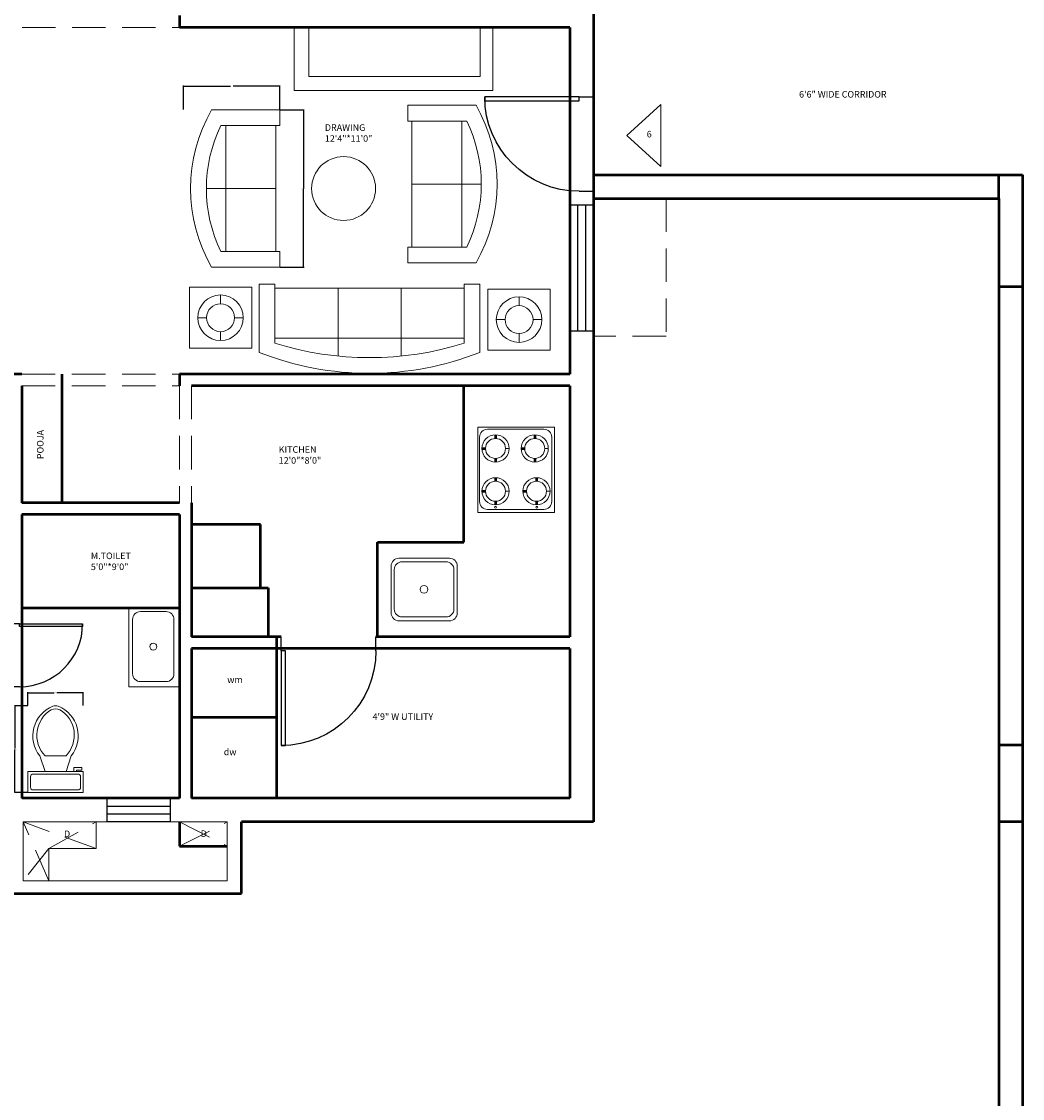
# Model space of a CAD drawing. Units: inches. Extents: x 4795 to 6024, y 2716 to 5025.
# Tile 10 of 19: x 5069 to 5450, y 3816 to 4226. Entities that reach past the tile are written whole.
import ezdxf

# ---------------------------------------------------------------- set-up
doc = ezdxf.new("R2010")
doc.units = ezdxf.units.IN
doc.linetypes.add('DASHED', pattern=[19.05, 12.7, -6.35])
for name, color, linetype, lineweight in [('A-ANNO-DIMS', 2, 'Continuous', 18), ('A-ANNO-TEXT', 7, 'Continuous', 18), ('A-AREA-IDEN', 3, 'Continuous', 18), ('A-DOOR', 4, 'Continuous', 25), ('A-FLOR-FIXT', 9, 'Continuous', 18), ('A-FURN', 8, 'Continuous', 18), ('A-GLAZ', 4, 'Continuous', 25), ('A-WALL', 7, 'Continuous', 50), ('A-WALL-OVHD', 8, 'DASHED', 18)]:
    doc.layers.add(name, color=color, linetype=linetype, lineweight=lineweight)
doc.styles.get("Standard").update_dxf_attribs({"font": 'arial.ttf'})
doc.dimstyles.get("Standard").update_dxf_attribs({"dimtxt": 0.18, "dimasz": 0.18, "dimexe": 0.18, "dimexo": 0.0625, "dimgap": 0.09, "dimtad": 0, "dimtih": 1, "dimtoh": 1, "dimdec": 4, "dimzin": 0, "dimdsep": 46, "dimtxsty": 'Standard', "dimcen": 0.09, "dimadec": 0, "dimazin": 0, "dimtfac": 1, "dimtdec": 4, "dimtofl": 0, "dimtmove": 0, "dimatfit": 3, "dimfxl": 1, "dimtolj": 1, "dimtzin": 0, "dimarcsym": 0})

# ---------------------------------------------------------------- blocks, each defined once
blk = doc.blocks.new('*U2')
for p, q in [((0, 0), (0, -6)), ((40, 0), (40, -6))]:
    blk.add_line(p, q)
blk.add_lwpolyline([(0, 0), (0, 40), (1.75, 40), (1.75, 0)], close=True)
blk.add_arc((0, 0), 40, 0, 90)
blk = doc.blocks.new('Toilet - top')
for p, q in [((9.5, -6), (9.5, -2)), ((-8, -8.5), (-8, -8)), ((-7, -8), (-7, -9.5)), ((-4, -8), (-6, -14)), ((4, -8), (6, -14)), ((-10, -8.5), (-8, -8.5)), ((-10, -9.5), (-10, -8.5)), ((-7, -9.5), (-10, -9.5)), ((4, -14), (-4, -14))]:
    blk.add_line(p, q)
blk.add_lwpolyline([(10.5, -8), (10.5, 0), (-10.5, 0), (-10.5, -8)], close=True)
for points in [[(-9.5, -2), (-9.5, -6)], [(8.5, -1), (-8.5, -1)], [(-8.5, -7), (8.5, -7)]]:
    blk.add_lwpolyline(points)
for centre, radius, start, end in [((-8.62, -1.88), 0.884, 81.8699, 188.1301), ((8.62, -1.88), 0.884, 351.8699, 98.1301), ((-8.62, -6.12), 0.884, 171.8699, 278.1301), ((8.62, -6.12), 0.884, 261.8699, 8.1301), ((3.52, -21.58), 12.17, 141.4691, 247.9714), ((4.2, -21.82), 11.33, 136.3677, 238.9468), ((-3.52, -21.58), 12.17, 292.0284, 38.5307), ((-4.2, -21.82), 11.33, 301.053, 43.6321), ((0, -27.88), 4, 245.7318, 294.2682), ((0, -29), 4, 254.8605, 285.1395)]:
    blk.add_arc(centre, radius, start, end)
blk = doc.blocks.new('Sofa - Roundback 7 ft.')
for p, q in [((-12.00002, -32.4421), (-12.00003, -6.5971)), ((11.99997, -32.4421), (11.99998, -6.5971)), ((-36.000027, -34), (-36.000027, -11.4696)), ((35.99998, -34), (35.99998, -11.4696)), ((-35.999844, -13.3819), (35.9998, -13.3819)), ((-36.000027, -32.4421), (35.99998, -32.4421))]:
    blk.add_line(p, q)
for points in [[(-36.000027, -34), (-42.000027, -34), (-42.000027, -8)], [(41.99998, -8), (41.99998, -34), (35.99998, -34)]]:
    blk.add_lwpolyline(points)
for centre, radius, start, end in [((0, -114.25), 114.25, 68.43141, 111.5686), ((-0.00001, -127.1968), 121.1968, 72.72033, 107.2797)]:
    blk.add_arc(centre, radius, start, end)
blk = doc.blocks.new('Sofa - Roundback Loveseat 5 ft.')
for p, q in [((0, -32.44198), (0, -5.99998)), ((-24, -33.99998), (-24, -11.46958)), ((24.00004, -33.99998), (24.00004, -11.46958)), ((-23.9998, -13.38178), (23.99986, -13.38178)), ((-24, -32.44198), (24.00004, -32.44198))]:
    blk.add_line(p, q)
for points in [[(-24, -33.99998), (-30, -33.99998), (-30, -7.99998)], [(30.00004, -7.99998), (30.00004, -33.99998), (24.00004, -33.99998)]]:
    blk.add_lwpolyline(points)
for centre, radius, start, end in [((0, -60.24998), 60.24998, 60.13715, 119.8628), ((0, -61.38438), 55.38444, 64.32083, 115.6792)]:
    blk.add_arc(centre, radius, start, end)
blk = doc.blocks.new('WIN-48')
for p, q in [((0, 0), (0, 48)), ((0, 48), (9, 48)), ((3, 0), (3, 48)), ((6, 48), (6, 0)), ((9, 48), (9, 0)), ((9, 0), (0, 0))]:
    blk.add_line(p, q)
blk = doc.blocks.new('WIN-24')
for p, q in [((0, 0), (0, 9)), ((0, 9), (24, 9)), ((24, 9), (24, 0)), ((0, 6), (24, 6)), ((24, 3), (0, 3)), ((24, 0), (0, 0))]:
    blk.add_line(p, q)
blk = doc.blocks.new('LAMP-SIDE')
for p, q in [((11.88, 20.25), (11.88, 16.92)), ((3.23, 11.6), (6.56, 11.6)), ((17.2, 11.6), (20.54, 11.6)), ((11.88, 6.28), (11.88, 2.94))]:
    blk.add_line(p, q)
blk.add_lwpolyline([(23.76, 23.19), (0, 23.19), (0, 0), (23.76, 0)], close=True)
for radius in [8.66, 5.32]:
    blk.add_circle((11.88, 11.6), radius)
blk = doc.blocks.new('*D27')
at = {"layer": 'A-ANNO-DIMS', "color": 0, "lineweight": -2, "transparency": 16777216}
for p, q in [((5071.7, 3965.06), (5066.63, 3965.06)), ((5066.81, 3964.88), (5066.81, 3948.72)), ((5066.81, 3932.19), (5066.81, 3948.35)), ((5071.7, 3932.01), (5066.63, 3932.01))]:
    blk.add_line(p, q, dxfattribs=at)
at = {"layer": 'A-ANNO-DIMS', "color": 0, "lineweight": 100, "transparency": 16777216}
for points in [[(5066.78, 3964.88), (5066.84, 3964.88), (5066.81, 3965.06)], [(5066.78, 3932.19), (5066.84, 3932.19), (5066.81, 3932.01)]]:
    blk.add_solid(points, dxfattribs=at)
at = {"layer": 'DEFPOINTS', "color": 0, "lineweight": 100, "transparency": 16777216}
for p in [(5071.76, 3965.06), (5066.81, 3932.01), (5071.76, 3932.01)]:
    blk.add_point(p, dxfattribs=at)
at = {"layer": 'A-ANNO-DIMS', "color": 0, "transparency": 16777216, "insert": (5066.81, 3948.53), "char_height": 0.18, "attachment_point": 5}
blk.add_mtext('\\A1;WC 33 TYP.', dxfattribs=at)
blk = doc.blocks.new('*D28')
at = {"layer": 'A-ANNO-DIMS', "color": 0, "lineweight": -2, "transparency": 16777216}
for p, q in [((5071.76, 3965.12), (5071.76, 3970.19)), ((5071.94, 3970.01), (5081.73, 3970.01)), ((5092.58, 3970.01), (5082.79, 3970.01)), ((5092.76, 3965.12), (5092.76, 3970.19))]:
    blk.add_line(p, q, dxfattribs=at)
at = {"layer": 'A-ANNO-DIMS', "color": 0, "lineweight": 100, "transparency": 16777216}
for points in [[(5071.94, 3970.04), (5071.94, 3969.98), (5071.76, 3970.01)], [(5092.58, 3970.04), (5092.58, 3969.98), (5092.76, 3970.01)]]:
    blk.add_solid(points, dxfattribs=at)
at = {"layer": 'DEFPOINTS', "color": 0, "lineweight": 100, "transparency": 16777216}
for p in [(5071.76, 3970.01), (5071.76, 3965.06), (5092.76, 3965.06)]:
    blk.add_point(p, dxfattribs=at)
at = {"layer": 'A-ANNO-DIMS', "color": 0, "transparency": 16777216, "insert": (5082.26, 3970.01), "char_height": 0.18, "attachment_point": 5}
blk.add_mtext('\\A1;21 TYP.', dxfattribs=at)
blk = doc.blocks.new('*D29')
at = {"layer": 'A-ANNO-DIMS', "color": 0, "lineweight": -2, "transparency": 16777216}
for p, q in [((5167.73, 4191.98), (5176.85, 4191.98)), ((5176.67, 4191.8), (5176.67, 4162.17)), ((5176.67, 4132.16), (5176.67, 4161.8)), ((5167.73, 4131.98), (5176.85, 4131.98))]:
    blk.add_line(p, q, dxfattribs=at)
at = {"layer": 'A-ANNO-DIMS', "color": 0, "lineweight": 100, "transparency": 16777216}
for points in [[(5176.64, 4191.8), (5176.7, 4191.8), (5176.67, 4191.98)], [(5176.64, 4132.16), (5176.7, 4132.16), (5176.67, 4131.98)]]:
    blk.add_solid(points, dxfattribs=at)
at = {"layer": 'DEFPOINTS', "color": 0, "lineweight": 100, "transparency": 16777216}
for p in [(5167.67, 4191.98), (5176.67, 4191.98), (5167.67, 4131.98)]:
    blk.add_point(p, dxfattribs=at)
at = {"layer": 'A-ANNO-DIMS', "color": 0, "transparency": 16777216, "insert": (5176.67, 4161.98), "char_height": 0.18, "attachment_point": 5}
blk.add_mtext('\\A1;LOVESEAT 60 TYP.', dxfattribs=at)
blk = doc.blocks.new('*D30')
at = {"layer": 'A-ANNO-DIMS', "color": 0, "lineweight": -2, "transparency": 16777216}
for p, q in [((5131, 4192.05), (5131, 4201.16)), ((5131.18, 4200.98), (5148.81, 4200.98)), ((5167.49, 4200.98), (5149.87, 4200.98)), ((5167.67, 4192.05), (5167.67, 4201.16))]:
    blk.add_line(p, q, dxfattribs=at)
at = {"layer": 'A-ANNO-DIMS', "color": 0, "lineweight": 100, "transparency": 16777216}
for points in [[(5131.18, 4201.01), (5131.18, 4200.95), (5131, 4200.98)], [(5167.49, 4201.01), (5167.49, 4200.95), (5167.67, 4200.98)]]:
    blk.add_solid(points, dxfattribs=at)
at = {"layer": 'DEFPOINTS', "color": 0, "lineweight": 100, "transparency": 16777216}
for p in [(5131, 4200.98), (5131, 4191.98), (5167.67, 4191.98)]:
    blk.add_point(p, dxfattribs=at)
at = {"layer": 'A-ANNO-DIMS', "color": 0, "transparency": 16777216, "insert": (5149.34, 4200.98), "char_height": 0.18, "attachment_point": 5}
blk.add_mtext('\\A1;37 TYP.', dxfattribs=at)

msp = doc.modelspace()

# ---------------------------------------------------------------- linework, layer by layer
at = {"layer": 'A-FLOR-FIXT'}
for points in [[(5242.93, 4071.13), (5272.17, 4071.13), (5272.17, 4038.61), (5242.93, 4038.61)], [(5129.47, 4002.32), (5110.15, 4002.32), (5110.15, 3972.27), (5129.47, 3972.27)]]:
    msp.add_lwpolyline(points, close=True, dxfattribs=at)
for points in [[(5246.65, 4070.33), (5268.11, 4070.33, -0.414214), (5271.11, 4067.33), (5271.11, 4042.79, -0.414214), (5268.11, 4039.79), (5246.65, 4039.79, -0.414214), (5243.65, 4042.79), (5243.65, 4067.33, -0.414214)], [(5212.95, 4021.19), (5232.16, 4021.19, -0.414214), (5235.16, 4018.19), (5235.16, 4000.39, -0.414214), (5232.16, 3997.39), (5212.95, 3997.39, -0.414214), (5209.95, 4000.39), (5209.95, 4018.19, -0.414214)], [(5214.15, 4019.88), (5230.88, 4019.88, -0.414214), (5233.88, 4016.88), (5233.88, 4001.86, -0.414214), (5230.88, 3998.86), (5214.15, 3998.86, -0.414214), (5211.15, 4001.86), (5211.15, 4016.88, -0.414214)], [(5114.61, 4000.9), (5124.34, 4000.9, -0.414214), (5127.34, 3997.9), (5127.34, 3977.25, -0.414214), (5124.34, 3974.25), (5114.61, 3974.25, -0.414214), (5111.61, 3977.25), (5111.61, 3997.9, -0.414214)]]:
    msp.add_lwpolyline(points, format="xyb", close=True, dxfattribs=at)
for centre, radius in [((5249.7, 4063.02), 5.16), ((5264.63, 4063.02), 5.16), ((5249.7, 4063.02), 3.8), ((5264.63, 4063.02), 3.8), ((5249.7, 4046.72), 5.16), ((5265.29, 4046.72), 5.16), ((5249.7, 4046.72), 3.8), ((5265.29, 4046.72), 3.8), ((5249.7, 4040.61), 0.353), ((5265.39, 4040.61), 0.353), ((5222.51, 4009.37), 1.48), ((5119.47, 3987.57), 1.3)]:
    msp.add_circle(centre, radius, dxfattribs=at)
at = {"layer": 'A-FURN'}
for p, q in [((5173.05, 4223.31), (5173.05, 4199.3)), ((5178.65, 4223.31), (5178.65, 4204.68)), ((5243.84, 4204.68), (5243.84, 4223.31)), ((5248.64, 4199.3), (5248.64, 4223.31)), ((5178.65, 4204.68), (5243.84, 4204.68)), ((5173.05, 4199.3), (5248.64, 4199.3)), ((5312.62, 4193.96), (5299.68, 4182.15)), ((5312.62, 4193.96), (5312.62, 4170.34)), ((5299.68, 4182.15), (5312.62, 4170.34)), ((5253.5, 4063.02), (5254.86, 4063.02)), ((5268.43, 4063.02), (5269.79, 4063.02)), ((5253.5, 4046.72), (5254.86, 4046.72)), ((5269.1, 4046.72), (5270.45, 4046.72)), ((5070, 3920.81), (5070, 3898.4)), ((5147.63, 3920.81), (5070, 3920.81)), ((5097.68, 3910.71), (5097.68, 3920.81)), ((5147.63, 3898.4), (5147.63, 3920.81)), ((5079.76, 3898.4), (5079.76, 3910.71)), ((5079.76, 3910.71), (5097.68, 3910.71)), ((5070, 3898.4), (5147.63, 3898.4))]:
    msp.add_line(p, q, dxfattribs=at)
msp.add_circle((5191.87, 4161.97), 12.16, dxfattribs=at)
at = {"layer": 'A-WALL'}
for p, q in [((5286.97, 4507.98), (5286.97, 4223.31)), ((5129.47, 4227.81), (5129.47, 4223.31)), ((5277.97, 4223.31), (5129.47, 4223.31)), ((5277.97, 4223.31), (5277.97, 4091.31)), ((5286.97, 4223.31), (5286.97, 3920.81)), ((5286.97, 4167.14), (5450.22, 4167.14)), ((5441.22, 4158.14), (5441.22, 4167.14)), ((5450.22, 4167.14), (5450.22, 3676.49)), ((5286.97, 4158.14), (5441.22, 4158.14)), ((5441.22, 4158.14), (5441.22, 3676.49)), ((5441.22, 4124.63), (5450.22, 4124.63)), ((5069.47, 4091.31), (5056.15, 4091.31)), ((5084.61, 4091.31), (5084.61, 4042.31)), ((5277.97, 4091.31), (5129.47, 4091.31)), ((5129.47, 4091.31), (5129.47, 4086.81)), ((5069.47, 4086.81), (5069.47, 4042.31)), ((5277.97, 4086.81), (5133.97, 4086.81)), ((5237.63, 4027.34), (5237.63, 4086.81)), ((5277.97, 4086.81), (5277.97, 3991.31)), ((5249.7, 4068.18), (5249.7, 4066.83)), ((5264.63, 4068.18), (5264.63, 4066.83)), ((5244.53, 4063.02), (5245.89, 4063.02)), ((5249.7, 4059.22), (5249.7, 4057.86)), ((5259.47, 4063.02), (5260.83, 4063.02)), ((5264.63, 4059.22), (5264.63, 4057.86)), ((5249.7, 4051.88), (5249.7, 4050.52)), ((5265.29, 4051.88), (5265.29, 4050.52)), ((5244.53, 4046.72), (5245.89, 4046.72)), ((5249.7, 4042.91), (5249.7, 4041.56)), ((5260.13, 4046.72), (5261.49, 4046.72)), ((5265.29, 4042.91), (5265.29, 4041.56)), ((5129.47, 4042.31), (5069.47, 4042.31)), ((5133.97, 4042.31), (5133.97, 3991.31)), ((5129.47, 4037.81), (5069.47, 4037.81)), ((5069.47, 4037.81), (5069.47, 3929.81)), ((5129.47, 4037.81), (5129.47, 3929.81)), ((5160.25, 4034.11), (5133.97, 4034.11)), ((5160.25, 4009.92), (5160.25, 4034.11)), ((5204.79, 3991.31), (5204.79, 4027.34)), ((5204.79, 4027.34), (5237.63, 4027.34)), ((5133.97, 4009.92), (5163.17, 4009.92)), ((5163.17, 4009.92), (5163.17, 3991.31)), ((5069.47, 4002.32), (5129.47, 4002.32)), ((5129.47, 4002.32), (5129.47, 4002.32)), ((5168.17, 3991.31), (5133.97, 3991.31)), ((5166.29, 3991.31), (5166.29, 3929.81)), ((5277.97, 3991.31), (5204.17, 3991.31)), ((5277.97, 3986.81), (5133.97, 3986.81)), ((5133.97, 3986.81), (5133.97, 3929.81)), ((5277.97, 3986.81), (5277.97, 3929.81)), ((5166.29, 3960.56), (5133.97, 3960.56)), ((5441.22, 3950.13), (5450.22, 3950.13)), ((5129.47, 3929.81), (5069.47, 3929.81)), ((5277.97, 3929.81), (5133.97, 3929.81)), ((5129.47, 3920.81), (5129.47, 3911.63)), ((5286.97, 3920.81), (5152.97, 3920.81)), ((5152.97, 3893.55), (5152.97, 3920.81)), ((5441.22, 3920.93), (5450.22, 3920.93)), ((5129.47, 3911.63), (5147.63, 3911.63)), ((5064.97, 3893.55), (5152.97, 3893.55))]:
    msp.add_line(p, q, dxfattribs=at)
at = {"layer": 'A-WALL-OVHD'}
for p, q in [((5050.47, 4223.31), (5129.47, 4223.31)), ((5286.97, 4158.17), (5314.58, 4158.17)), ((5314.58, 4158.17), (5314.58, 4105.81)), ((5314.58, 4105.81), (5286.97, 4105.81)), ((5069.47, 4091.31), (5129.47, 4091.31)), ((5069.47, 4086.81), (5129.47, 4086.81)), ((5129.47, 4086.81), (5129.47, 4042.31)), ((5133.97, 4086.81), (5133.97, 4042.31)), ((5097.68, 3910.71), (5070, 3920.81)), ((5079.76, 3898.4), (5070, 3920.81)), ((5079.76, 3910.71), (5097.68, 3920.81)), ((5129.47, 3920.81), (5147.63, 3911.63)), ((5129.47, 3911.63), (5147.63, 3920.81)), ((5079.76, 3910.71), (5070, 3898.4))]:
    msp.add_line(p, q, dxfattribs=at)

# ---------------------------------------------------------------- block references
at = {"layer": 'A-DOOR'}
for p, xscale, yscale, zscale, rotation in [((5281.57, 4196.94), -0.9, 0.9, 0.9, 90), ((5068.57, 3996.29), 0.6, 0.6, 0.6, 270), ((5168.17, 3985.91), -0.9, 0.9, 0.9, 180)]:
    msp.add_blockref('*U2', p, dxfattribs=dict(at, xscale=xscale, yscale=yscale, zscale=zscale, rotation=rotation))
at = {"layer": 'A-FLOR-FIXT', "rotation": 180}
msp.add_blockref('Toilet - top', (5082.26, 3932.01), dxfattribs=at)
at = {"layer": 'A-FURN'}
for name, p, rotation in [('Sofa - Roundback Loveseat 5 ft.', (5133.67, 4161.98), 90), ('Sofa - Roundback Loveseat 5 ft.', (5250.27, 4163.68), 270), ('Sofa - Roundback 7 ft.', (5201.77, 4091.6), 180)]:
    msp.add_blockref(name, p, dxfattribs=dict(at, rotation=rotation))
for p in [(5133.18, 4101.19), (5246.78, 4100.48)]:
    msp.add_blockref('LAMP-SIDE', p, dxfattribs=at)
at = {"layer": 'A-GLAZ', "rotation": 180}
for name, p in [('WIN-48', (5286.97, 4155.73)), ('WIN-24', (5125.88, 3929.81))]:
    msp.add_blockref(name, p, dxfattribs=at)

# ---------------------------------------------------------------- texts
at = {"layer": 'A-ANNO-TEXT', "char_height": 2.5, "attachment_point": 1}
for s, width, insert in [('6', 6.0367, (5307.24, 4183.93)), ('wm', 14.6182, (5147.62, 3976.22)), ('dw', 9.6121, (5146.28, 3948.74)), ('D', 2.5035, (5085.49, 3917.54)), ('D', 1.7777, (5137.51, 3917.61))]:
    msp.add_mtext_dynamic_manual_height_columns(s, width=width, gutter_width=12.5, heights=[0], dxfattribs=dict(at, insert=insert))
at = {"layer": 'A-AREA-IDEN', "char_height": 2.5, "attachment_point": 1}
for s, width, insert in [('6\'6" WIDE CORRIDOR', 101.5124, (5365.22, 4199.1)), ('DRAWING\\P12\'4"*11\'0"', 32.8206, (5184.75, 4186.44)), ('KITCHEN\\P12\'0"*8\'0"', 51.8096, (5167.19, 4063.87)), ('M.TOILET\\P5\'0"*9\'0"', 43.2093, (5095.71, 4023.38)), ('4\'9" W UTILITY', 65.4529, (5202.9, 3962.15))]:
    msp.add_mtext_dynamic_manual_height_columns(s, width=width, gutter_width=12.5, heights=[0], dxfattribs=dict(at, insert=insert))
at = {"layer": 'A-AREA-IDEN', "insert": (5075.19, 4058.95), "char_height": 2.5, "attachment_point": 1, "rotation": 90}
msp.add_mtext_dynamic_manual_height_columns('POOJA', width=11.474, gutter_width=12.5, heights=[0], dxfattribs=at)

# ---------------------------------------------------------------- dimensions: what is measured, and where the dimension line sits
at = {"layer": 'A-ANNO-DIMS'}
for base, p1, p2, angle, text, picture, middle in [((5131, 4200.98), (5167.67, 4191.98), (5131, 4191.98), 180, '<> TYP.', '*D30', (5149.34, 4200.98)), ((5176.67, 4191.98), (5167.67, 4131.98), (5167.67, 4191.98), 90, 'LOVESEAT <> TYP.', '*D29', (5176.67, 4161.98)), ((5071.76, 3970.01), (5092.76, 3965.06), (5071.76, 3965.06), 180, '<> TYP.', '*D28', (5082.26, 3970.01)), ((5066.81, 3932.01), (5071.76, 3965.06), (5071.76, 3932.01), 270, 'WC <> TYP.', '*D27', (5066.81, 3948.53))]:
    dim = msp.add_linear_dim(base=base, p1=p1, p2=p2, angle=angle, text=text, dimstyle='Standard', override={"dimdec": 0, "dimlfac": 1, "dimrnd": 0, "dimzin": 0, "dimdsep": 46, "dimlunit": 2}, dxfattribs=at)
    dim.commit()
    dim.dimension.update_dxf_attribs({"geometry": picture, "text_midpoint": middle})

doc.saveas('drawing.dxf')
